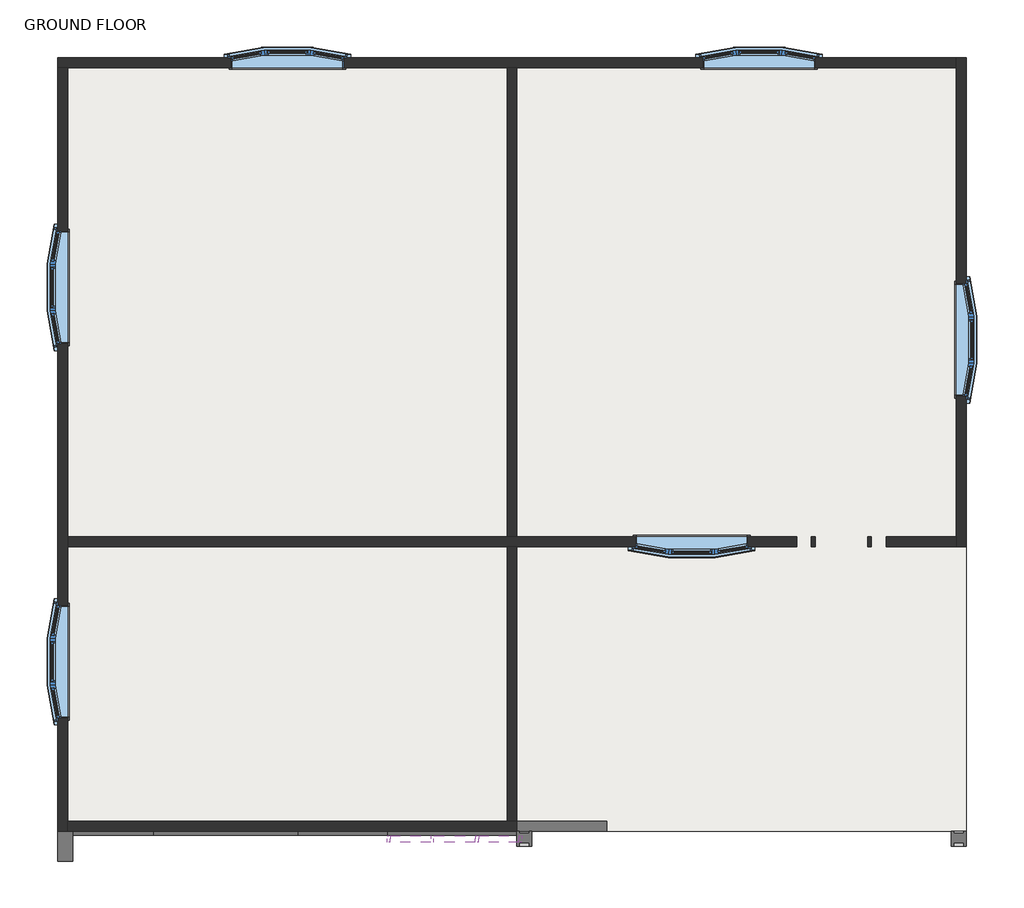
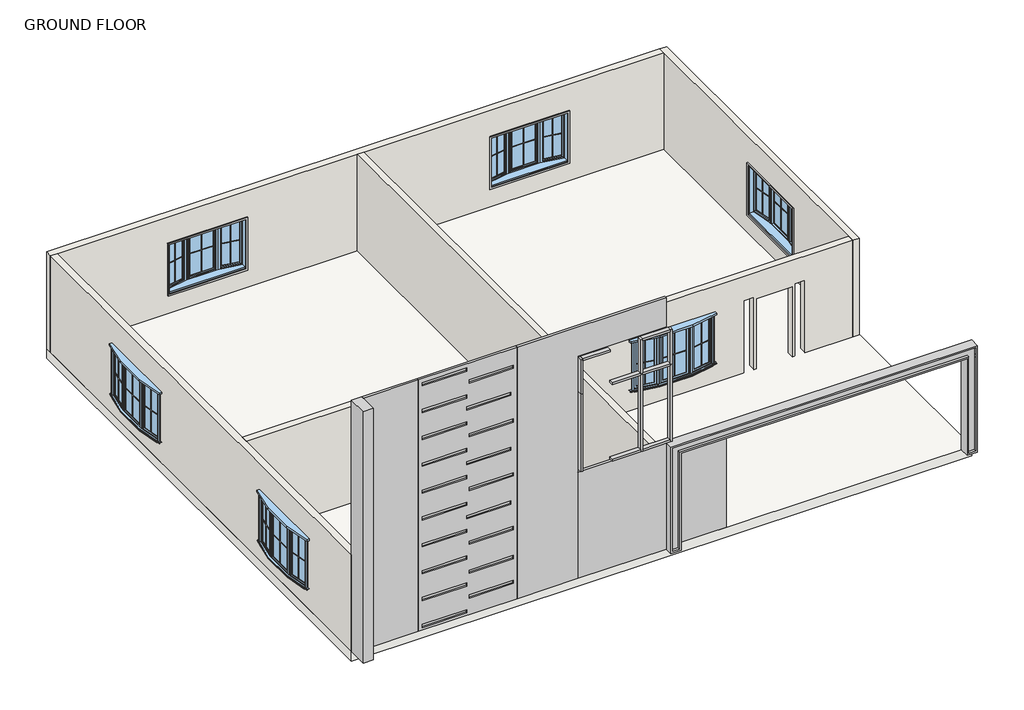
# One storey, incomplete: 31 proxies, 12 members, 7 walls, 6 windows, 1 slab.
"""IFC4 building model written with IfcOpenShell, lengths in millimetres."""

from ifc_helpers import new_model, si_unit, frame, origin, origin_with_axes, place, context, project, spatial, polyline, outline, extrude, faceted_brep, transform, mapped, element, save
from components import generic_models_1_generic_models_1_d450fbd8, generic_models_3_generic_models_3_9b1755e3, generic_models_4_generic_models_4_91b2e968, generic_models_5_generic_models_5_f46b040b, generic_models_6_generic_models_6_d33aa09a, generic_models_7_generic_models_7_539d4222, generic_models_8_generic_models_8_98324a9d, muntin_pattern_2x2_muntin_pattern_2x2_d8607f27, muntin_pattern_2x2_muntin_pattern_2x2_395d1e8c, trim_window_interior_flat_picture_frame_9ca7b173, member_f0fea5a5, member_ee409385, member_b90701c7, member_3972cc06, member_bef5179f, member_a085fe98, member_9b18e963, member_95153237, window_3790adff

model = new_model("IFC4")

# Units and contexts
model_context = context("Model", 3, world=origin())
ifc_project = project(units=[si_unit("LENGTHUNIT", "METRE", prefix="MILLI")], contexts=[model_context])

# Site, building, storey
site = spatial("IfcSite", under=ifc_project)
building = spatial("IfcBuilding", under=site)
storey = spatial("IfcBuildingStorey", under=building, Name="GROUND FLOOR", Elevation=0.0)

# Proxies
placement = place(None, origin())
generic_models_1_generic_models_1_shape = generic_models_1_generic_models_1_d450fbd8(model_context)
element("IfcBuildingElementProxy", 1, Name="Generic Models 1 : Generic Models 1", ObjectType="Generic Models 1 : Generic Models 1", at=placement, inside=storey, context=model_context, shape_type="MappedRepresentation", body=[
    mapped(generic_models_1_generic_models_1_shape, transform((0.0, 0.0, 0.0), x_axis=(1.0, 0.0, 0.0), y_axis=(0.0, 1.0, 0.0), z_axis=(0.0, 0.0, 1.0))),
])
generic_models_3_generic_models_3_shape = generic_models_3_generic_models_3_9b1755e3(model_context)
element("IfcBuildingElementProxy", 2, Name="Generic Models 3 : Generic Models 3", ObjectType="Generic Models 3 : Generic Models 3", at=placement, inside=storey, context=model_context, shape_type="MappedRepresentation", body=[
    mapped(generic_models_3_generic_models_3_shape, transform((0.0, 0.0, 0.0), x_axis=(1.0, 0.0, 0.0), y_axis=(0.0, 1.0, 0.0), z_axis=(0.0, 0.0, 1.0))),
])
generic_models_4_generic_models_4_shape = generic_models_4_generic_models_4_91b2e968(model_context)
element("IfcBuildingElementProxy", 3, Name="Generic Models 4 : Generic Models 4", ObjectType="Generic Models 4 : Generic Models 4", at=placement, inside=storey, context=model_context, shape_type="MappedRepresentation", body=[
    mapped(generic_models_4_generic_models_4_shape, transform((0.0, 0.0, 0.0), x_axis=(1.0, 0.0, 0.0), y_axis=(0.0, 1.0, 0.0), z_axis=(0.0, 0.0, 1.0))),
])
generic_models_5_generic_models_5_shape = generic_models_5_generic_models_5_f46b040b(model_context)
element("IfcBuildingElementProxy", 4, Name="Generic Models 5 : Generic Models 5", ObjectType="Generic Models 5 : Generic Models 5", at=placement, inside=storey, context=model_context, shape_type="MappedRepresentation", body=[
    mapped(generic_models_5_generic_models_5_shape, transform((0.0, 0.0, 0.0), x_axis=(1.0, 0.0, 0.0), y_axis=(0.0, 1.0, 0.0), z_axis=(0.0, 0.0, 1.0))),
])
generic_models_6_generic_models_6_shape = generic_models_6_generic_models_6_d33aa09a(model_context)
element("IfcBuildingElementProxy", 5, Name="Generic Models 6 : Generic Models 6", ObjectType="Generic Models 6 : Generic Models 6", at=placement, inside=storey, context=model_context, shape_type="MappedRepresentation", body=[
    mapped(generic_models_6_generic_models_6_shape, transform((0.0, 0.0, 0.0), x_axis=(1.0, 0.0, 0.0), y_axis=(0.0, 1.0, 0.0), z_axis=(0.0, 0.0, 1.0))),
])
generic_models_7_generic_models_7_shape = generic_models_7_generic_models_7_539d4222(model_context)
element("IfcBuildingElementProxy", 6, Name="Generic Models 7 : Generic Models 7", ObjectType="Generic Models 7 : Generic Models 7", at=placement, inside=storey, context=model_context, shape_type="MappedRepresentation", body=[
    mapped(generic_models_7_generic_models_7_shape, transform((0.0, 0.0, 0.0), x_axis=(1.0, 0.0, 0.0), y_axis=(0.0, 1.0, 0.0), z_axis=(0.0, 0.0, 1.0))),
])
generic_models_8_generic_models_8_shape = generic_models_8_generic_models_8_98324a9d(model_context)
element("IfcBuildingElementProxy", 7, Name="Generic Models 8 : Generic Models 8", ObjectType="Generic Models 8 : Generic Models 8", at=placement, inside=storey, context=model_context, shape_type="MappedRepresentation", body=[
    mapped(generic_models_8_generic_models_8_shape, transform((0.0, 0.0, 0.0), x_axis=(1.0, 0.0, 0.0), y_axis=(0.0, 1.0, 0.0), z_axis=(0.0, 0.0, 1.0))),
])
muntin_pattern_2x2_muntin_pattern_2x2_shape = muntin_pattern_2x2_muntin_pattern_2x2_d8607f27(model_context)
element("IfcBuildingElementProxy", 8, Name="Muntin Pattern_2x2 : Muntin Pattern_2x2", ObjectType="Muntin Pattern_2x2 : Muntin Pattern_2x2", at=placement, inside=storey, context=model_context, shape_type="MappedRepresentation", body=[
    mapped(muntin_pattern_2x2_muntin_pattern_2x2_shape, transform((4145.554407, 1568.600611, 730.25), x_axis=(-1.0, 0.0, 0.0), y_axis=(0.0, -1.0, 0.0), z_axis=(0.0, 0.0, 1.0))),
])
element("IfcBuildingElementProxy", 9, Name="Muntin Pattern_2x2 : Muntin Pattern_2x2", ObjectType="Muntin Pattern_2x2 : Muntin Pattern_2x2", at=placement, inside=storey, context=model_context, shape_type="MappedRepresentation", body=[
    mapped(muntin_pattern_2x2_muntin_pattern_2x2_shape, transform((9844.679407, 5896.125611, 730.25), x_axis=(0.0, -1.0, 0.0), y_axis=(1.0, 0.0, 0.0), z_axis=(0.0, 0.0, 1.0))),
])
element("IfcBuildingElementProxy", 10, Name="Muntin Pattern_2x2 : Muntin Pattern_2x2", ObjectType="Muntin Pattern_2x2 : Muntin Pattern_2x2", at=placement, inside=storey, context=model_context, shape_type="MappedRepresentation", body=[
    mapped(muntin_pattern_2x2_muntin_pattern_2x2_shape, transform((-4084.045593, 11747.650611, 730.25), x_axis=(1.0, 0.0, 0.0), y_axis=(0.0, 1.0, 0.0), z_axis=(0.0, 0.0, 1.0))),
])
element("IfcBuildingElementProxy", 11, Name="Muntin Pattern_2x2 : Muntin Pattern_2x2", ObjectType="Muntin Pattern_2x2 : Muntin Pattern_2x2", at=placement, inside=storey, context=model_context, shape_type="MappedRepresentation", body=[
    mapped(muntin_pattern_2x2_muntin_pattern_2x2_shape, transform((5517.154407, 11747.650611, 730.25), x_axis=(1.0, 0.0, 0.0), y_axis=(0.0, 1.0, 0.0), z_axis=(0.0, 0.0, 1.0))),
])
element("IfcBuildingElementProxy", 12, Name="Muntin Pattern_2x2 : Muntin Pattern_2x2", ObjectType="Muntin Pattern_2x2 : Muntin Pattern_2x2", at=placement, inside=storey, context=model_context, shape_type="MappedRepresentation", body=[
    mapped(muntin_pattern_2x2_muntin_pattern_2x2_shape, transform((-8868.770593, 6962.925611, 730.25), x_axis=(0.0, 1.0, 0.0), y_axis=(-1.0, 0.0, 0.0), z_axis=(0.0, 0.0, 1.0))),
])
element("IfcBuildingElementProxy", 13, Name="Muntin Pattern_2x2 : Muntin Pattern_2x2", ObjectType="Muntin Pattern_2x2 : Muntin Pattern_2x2", at=placement, inside=storey, context=model_context, shape_type="MappedRepresentation", body=[
    mapped(muntin_pattern_2x2_muntin_pattern_2x2_shape, transform((-8868.770593, -657.074389, 730.25), x_axis=(0.0, 1.0, 0.0), y_axis=(-1.0, 0.0, 0.0), z_axis=(0.0, 0.0, 1.0))),
])
muntin_pattern_2x2_muntin_pattern_2x2_2_shape = muntin_pattern_2x2_muntin_pattern_2x2_395d1e8c(model_context)
element("IfcBuildingElementProxy", 14, Name="Muntin Pattern_2x2 : Muntin Pattern_2x2", ObjectType="Muntin Pattern_2x2 : Muntin Pattern_2x2", at=placement, inside=storey, context=model_context, shape_type="MappedRepresentation", body=[
    mapped(muntin_pattern_2x2_muntin_pattern_2x2_2_shape, transform((4981.9237745, 1633.1915685, 730.25), x_axis=(-0.9848077530122097, -0.1736481776669209, 0.0), y_axis=(0.1736481776669209, -0.9848077530122097, 0.0), z_axis=(0.0, 0.0, 1.0))),
])
element("IfcBuildingElementProxy", 15, Name="Muntin Pattern_2x2 : Muntin Pattern_2x2", ObjectType="Muntin Pattern_2x2 : Muntin Pattern_2x2", at=placement, inside=storey, context=model_context, shape_type="MappedRepresentation", body=[
    mapped(muntin_pattern_2x2_muntin_pattern_2x2_2_shape, transform((3309.1850396, 1633.1915685, 730.25), x_axis=(-0.9848077530122065, 0.17364817766693977, 0.0), y_axis=(-0.17364817766693977, -0.9848077530122065, 0.0), z_axis=(0.0, 0.0, 1.0))),
])
element("IfcBuildingElementProxy", 16, Name="Muntin Pattern_2x2 : Muntin Pattern_2x2", ObjectType="Muntin Pattern_2x2 : Muntin Pattern_2x2", at=placement, inside=storey, context=model_context, shape_type="MappedRepresentation", body=[
    mapped(muntin_pattern_2x2_muntin_pattern_2x2_2_shape, transform((9780.0884495, 6732.4949785, 730.25), x_axis=(0.1736481776669241, -0.9848077530122091, 0.0), y_axis=(0.9848077530122091, 0.1736481776669241, 0.0), z_axis=(0.0, 0.0, 1.0))),
])
element("IfcBuildingElementProxy", 17, Name="Muntin Pattern_2x2 : Muntin Pattern_2x2", ObjectType="Muntin Pattern_2x2 : Muntin Pattern_2x2", at=placement, inside=storey, context=model_context, shape_type="MappedRepresentation", body=[
    mapped(muntin_pattern_2x2_muntin_pattern_2x2_2_shape, transform((9780.0884495, 5059.7562435, 730.25), x_axis=(-0.17364817766693658, -0.984807753012207, 0.0), y_axis=(0.984807753012207, -0.17364817766693658, 0.0), z_axis=(0.0, 0.0, 1.0))),
])
element("IfcBuildingElementProxy", 18, Name="Muntin Pattern_2x2 : Muntin Pattern_2x2", ObjectType="Muntin Pattern_2x2 : Muntin Pattern_2x2", at=placement, inside=storey, context=model_context, shape_type="MappedRepresentation", body=[
    mapped(muntin_pattern_2x2_muntin_pattern_2x2_2_shape, transform((-4920.4149604, 11683.0596534, 730.25), x_axis=(0.9848077530122091, 0.1736481776669241, 0.0), y_axis=(-0.1736481776669241, 0.9848077530122091, 0.0), z_axis=(0.0, 0.0, 1.0))),
])
element("IfcBuildingElementProxy", 19, Name="Muntin Pattern_2x2 : Muntin Pattern_2x2", ObjectType="Muntin Pattern_2x2 : Muntin Pattern_2x2", at=placement, inside=storey, context=model_context, shape_type="MappedRepresentation", body=[
    mapped(muntin_pattern_2x2_muntin_pattern_2x2_2_shape, transform((-3247.6762255, 11683.0596534, 730.25), x_axis=(0.984807753012207, -0.17364817766693658, 0.0), y_axis=(0.17364817766693658, 0.984807753012207, 0.0), z_axis=(0.0, 0.0, 1.0))),
])
element("IfcBuildingElementProxy", 20, Name="Muntin Pattern_2x2 : Muntin Pattern_2x2", ObjectType="Muntin Pattern_2x2 : Muntin Pattern_2x2", at=placement, inside=storey, context=model_context, shape_type="MappedRepresentation", body=[
    mapped(muntin_pattern_2x2_muntin_pattern_2x2_2_shape, transform((4680.7850396, 11683.0596534, 730.25), x_axis=(0.9848077530122091, 0.1736481776669241, 0.0), y_axis=(-0.1736481776669241, 0.9848077530122091, 0.0), z_axis=(0.0, 0.0, 1.0))),
])
element("IfcBuildingElementProxy", 21, Name="Muntin Pattern_2x2 : Muntin Pattern_2x2", ObjectType="Muntin Pattern_2x2 : Muntin Pattern_2x2", at=placement, inside=storey, context=model_context, shape_type="MappedRepresentation", body=[
    mapped(muntin_pattern_2x2_muntin_pattern_2x2_2_shape, transform((6353.5237745, 11683.0596534, 730.25), x_axis=(0.984807753012207, -0.17364817766693658, 0.0), y_axis=(0.17364817766693658, 0.984807753012207, 0.0), z_axis=(0.0, 0.0, 1.0))),
])
element("IfcBuildingElementProxy", 22, Name="Muntin Pattern_2x2 : Muntin Pattern_2x2", ObjectType="Muntin Pattern_2x2 : Muntin Pattern_2x2", at=placement, inside=storey, context=model_context, shape_type="MappedRepresentation", body=[
    mapped(muntin_pattern_2x2_muntin_pattern_2x2_2_shape, transform((-8804.1796354, 6126.5562435, 730.25), x_axis=(-0.1736481776669241, 0.9848077530122091, 0.0), y_axis=(-0.9848077530122091, -0.1736481776669241, 0.0), z_axis=(0.0, 0.0, 1.0))),
])
element("IfcBuildingElementProxy", 23, Name="Muntin Pattern_2x2 : Muntin Pattern_2x2", ObjectType="Muntin Pattern_2x2 : Muntin Pattern_2x2", at=placement, inside=storey, context=model_context, shape_type="MappedRepresentation", body=[
    mapped(muntin_pattern_2x2_muntin_pattern_2x2_2_shape, transform((-8804.1796354, 7799.2949785, 730.25), x_axis=(0.17364817766693658, 0.984807753012207, 0.0), y_axis=(-0.984807753012207, 0.17364817766693658, 0.0), z_axis=(0.0, 0.0, 1.0))),
])
element("IfcBuildingElementProxy", 24, Name="Muntin Pattern_2x2 : Muntin Pattern_2x2", ObjectType="Muntin Pattern_2x2 : Muntin Pattern_2x2", at=placement, inside=storey, context=model_context, shape_type="MappedRepresentation", body=[
    mapped(muntin_pattern_2x2_muntin_pattern_2x2_2_shape, transform((-8804.1796354, -1493.4437565, 730.25), x_axis=(-0.1736481776669241, 0.9848077530122091, 0.0), y_axis=(-0.9848077530122091, -0.1736481776669241, 0.0), z_axis=(0.0, 0.0, 1.0))),
])
element("IfcBuildingElementProxy", 25, Name="Muntin Pattern_2x2 : Muntin Pattern_2x2", ObjectType="Muntin Pattern_2x2 : Muntin Pattern_2x2", at=placement, inside=storey, context=model_context, shape_type="MappedRepresentation", body=[
    mapped(muntin_pattern_2x2_muntin_pattern_2x2_2_shape, transform((-8804.1796354, 179.2949785, 730.25), x_axis=(0.17364817766693658, 0.984807753012207, 0.0), y_axis=(-0.984807753012207, 0.17364817766693658, 0.0), z_axis=(0.0, 0.0, 1.0))),
])
trim_window_interior_flat_picture_frame_shape = trim_window_interior_flat_picture_frame_9ca7b173(model_context)
element("IfcBuildingElementProxy", 26, Name="Trim-Window-Interior-Flat : Picture Frame", ObjectType="Trim-Window-Interior-Flat : Picture Frame", at=placement, inside=storey, context=model_context, shape_type="MappedRepresentation", body=[
    mapped(trim_window_interior_flat_picture_frame_shape, transform((4145.554407, 1882.925611, 2184.4), x_axis=(-1.0, 0.0, 0.0), y_axis=(0.0, 0.0, 1.0), z_axis=(0.0, 1.0, 0.0))),
])
element("IfcBuildingElementProxy", 27, Name="Trim-Window-Interior-Flat : Picture Frame", ObjectType="Trim-Window-Interior-Flat : Picture Frame", at=placement, inside=storey, context=model_context, shape_type="MappedRepresentation", body=[
    mapped(trim_window_interior_flat_picture_frame_shape, transform((9530.354407, 5896.125611, 2184.4), x_axis=(0.0, -1.0, 0.0), y_axis=(0.0, 0.0, 1.0), z_axis=(-1.0, 0.0, 0.0))),
])
element("IfcBuildingElementProxy", 28, Name="Trim-Window-Interior-Flat : Picture Frame", ObjectType="Trim-Window-Interior-Flat : Picture Frame", at=placement, inside=storey, context=model_context, shape_type="MappedRepresentation", body=[
    mapped(trim_window_interior_flat_picture_frame_shape, transform((-4084.045593, 11433.325611, 2184.4), x_axis=(1.0, 0.0, 0.0), y_axis=(0.0, 0.0, 1.0), z_axis=(0.0, -1.0, 0.0))),
])
element("IfcBuildingElementProxy", 29, Name="Trim-Window-Interior-Flat : Picture Frame", ObjectType="Trim-Window-Interior-Flat : Picture Frame", at=placement, inside=storey, context=model_context, shape_type="MappedRepresentation", body=[
    mapped(trim_window_interior_flat_picture_frame_shape, transform((5517.154407, 11433.325611, 2184.4), x_axis=(1.0, 0.0, 0.0), y_axis=(0.0, 0.0, 1.0), z_axis=(0.0, -1.0, 0.0))),
])
element("IfcBuildingElementProxy", 30, Name="Trim-Window-Interior-Flat : Picture Frame", ObjectType="Trim-Window-Interior-Flat : Picture Frame", at=placement, inside=storey, context=model_context, shape_type="MappedRepresentation", body=[
    mapped(trim_window_interior_flat_picture_frame_shape, transform((-8554.445593, 6962.925611, 2184.4), x_axis=(0.0, 1.0, 0.0), y_axis=(0.0, 0.0, 1.0), z_axis=(1.0, 0.0, 0.0))),
])
element("IfcBuildingElementProxy", 31, Name="Trim-Window-Interior-Flat : Picture Frame", ObjectType="Trim-Window-Interior-Flat : Picture Frame", at=placement, inside=storey, context=model_context, shape_type="MappedRepresentation", body=[
    mapped(trim_window_interior_flat_picture_frame_shape, transform((-8554.445593, -657.074389, 2184.4), x_axis=(0.0, 1.0, 0.0), y_axis=(0.0, 0.0, 1.0), z_axis=(1.0, 0.0, 0.0))),
])

# Members
member_shape = member_f0fea5a5(model_context)
element("IfcMember", 32, ObjectType="Rectangular Mullion : 2.5\" x 5\" rectangular", at=placement, inside=storey, context=model_context, shape_type="MappedRepresentation", body=[
    mapped(member_shape, transform((-223.2455734, -4263.874389, 3450.2081328), x_axis=(-1.0, 0.0, 0.0), y_axis=(0.0, 1.0, 0.0), z_axis=(0.0, 0.0, -1.0))),
])
member_2_shape = member_ee409385(model_context)
element("IfcMember", 33, ObjectType="Rectangular Mullion : 2.5\" x 5\" rectangular", at=placement, inside=storey, context=model_context, shape_type="MappedRepresentation", body=[
    mapped(member_2_shape, transform((-2052.0455733, -4263.874389, 3450.2081328), x_axis=(-1.0, 0.0, 0.0), y_axis=(0.0, 1.0, 0.0), z_axis=(0.0, 0.0, -1.0))),
])
element("IfcMember", 34, ObjectType="Rectangular Mullion : 2.5\" x 5\" rectangular", at=placement, inside=storey, context=model_context, shape_type="MappedRepresentation", body=[
    mapped(member_2_shape, transform((691.1544267, -4263.874389, 5888.6081328), x_axis=(1.0, 0.0, 0.0), y_axis=(0.0, 1.0, 0.0), z_axis=(0.0, 0.0, 1.0))),
])
member_3_shape = member_b90701c7(model_context)
element("IfcMember", 35, ObjectType="Rectangular Mullion : 2.5\" x 5\" rectangular", at=placement, inside=storey, context=model_context, shape_type="MappedRepresentation", body=[
    mapped(member_3_shape, transform((-223.2455734, -4263.874389, 5888.6081328), x_axis=(-1.0, 0.0, 0.0), y_axis=(0.0, 1.0, 0.0), z_axis=(0.0, 0.0, -1.0))),
])
member_4_shape = member_3972cc06(model_context)
element("IfcMember", 36, ObjectType="Rectangular Mullion : 2.5\" x 5\" rectangular", at=placement, inside=storey, context=model_context, shape_type="MappedRepresentation", body=[
    mapped(member_4_shape, transform((-2052.0455733, -4263.874389, 5888.6081328), x_axis=(-1.0, 0.0, 0.0), y_axis=(0.0, 1.0, 0.0), z_axis=(0.0, 0.0, -1.0))),
])
element("IfcMember", 37, ObjectType="Rectangular Mullion : 2.5\" x 5\" rectangular", at=placement, inside=storey, context=model_context, shape_type="MappedRepresentation", body=[
    mapped(member_4_shape, transform((691.1544267, -4263.874389, 6988.1851727), x_axis=(1.0, 0.0, 0.0), y_axis=(0.0, 1.0, 0.0), z_axis=(0.0, 0.0, 1.0))),
])
member_5_shape = member_bef5179f(model_context)
element("IfcMember", 38, ObjectType="Rectangular Mullion : 2.5\" x 5\" rectangular", at=placement, inside=storey, context=model_context, shape_type="MappedRepresentation", body=[
    mapped(member_5_shape, transform((-1988.5455733, -4263.874389, 6988.1851727), x_axis=(0.0, 0.0, 1.0), y_axis=(0.0, 1.0, 0.0), z_axis=(-1.0, 0.0, 0.0))),
])
element("IfcMember", 39, ObjectType="Rectangular Mullion : 2.5\" x 5\" rectangular", at=placement, inside=storey, context=model_context, shape_type="MappedRepresentation", body=[
    mapped(member_5_shape, transform((-191.4955734, -4263.874389, 6988.1851727), x_axis=(0.0, 0.0, 1.0), y_axis=(0.0, 1.0, 0.0), z_axis=(-1.0, 0.0, 0.0))),
])
element("IfcMember", 40, ObjectType="Rectangular Mullion : 2.5\" x 5\" rectangular", at=placement, inside=storey, context=model_context, shape_type="MappedRepresentation", body=[
    mapped(member_5_shape, transform((627.6544267, -4263.874389, 3450.2081328), x_axis=(0.0, 0.0, -1.0), y_axis=(0.0, 1.0, 0.0), z_axis=(1.0, 0.0, 0.0))),
])
member_6_shape = member_a085fe98(model_context)
element("IfcMember", 41, ObjectType="Rectangular Mullion : 2.5\" x 5\" rectangular", at=placement, inside=storey, context=model_context, shape_type="MappedRepresentation", body=[
    mapped(member_6_shape, transform((-191.4955734, -4263.874389, 5888.6081328), x_axis=(0.0, 0.0, 1.0), y_axis=(0.0, 1.0, 0.0), z_axis=(-1.0, 0.0, 0.0))),
])
member_7_shape = member_9b18e963(model_context)
element("IfcMember", 42, ObjectType="Rectangular Mullion : 2.5\" x 5\" rectangular", at=placement, inside=storey, context=model_context, shape_type="MappedRepresentation", body=[
    mapped(member_7_shape, transform((-254.9955734, -4263.874389, 3450.2081328), x_axis=(0.0, 0.0, -1.0), y_axis=(0.0, 1.0, 0.0), z_axis=(1.0, 0.0, 0.0))),
])
member_8_shape = member_95153237(model_context)
element("IfcMember", 43, ObjectType="Rectangular Mullion : 2.5\" x 5\" rectangular", at=placement, inside=storey, context=model_context, shape_type="MappedRepresentation", body=[
    mapped(member_8_shape, transform((-1105.8955732, -4263.874389, 5888.6081328), x_axis=(0.0, 0.0, 1.0), y_axis=(0.0, 1.0, 0.0), z_axis=(-1.0, 0.0, 0.0))),
])

# Slab
element("IfcSlab", 44, ObjectType="Generic - 12\"", at=placement, inside=storey, context=model_context, shape_type="SweptSolid", body=[
    extrude(outline(polyline([(9733.554407, 11636.525611), (9733.554407, -4111.474389), (-8757.645593, -4111.474389), (-8757.645593, 11636.525611), (9733.554407, 11636.525611)])), frame((0.0, 0.0, -304.8), z_axis=(0.0, 0.0, 1.0), x_axis=(1.0, 0.0, 0.0)), (0.0, 0.0, 1.0), 304.8),
])

# Walls
element("IfcWall", 45, ObjectType="Generic - 8\"", at=placement, inside=storey, context=model_context, shape_type="Brep", body=[
    faceted_brep([(-8757.645593, 11433.325611, 0.0), (-8554.445593, 11433.325611, 0.0), (386.354407, 11433.325611, 0.0), (589.554407, 11433.325611, 0.0), (9530.354407, 11433.325611, 0.0), (9530.354407, 11433.325611, 3048.0), (589.554407, 11433.325611, 3048.0), (386.354407, 11433.325611, 3048.0), (-8554.445593, 11433.325611, 3048.0), (-8757.645593, 11433.325611, 3048.0), (-5227.045593, 11433.325611, 2184.4), (-2941.045593, 11433.325611, 2184.4), (-2941.045593, 11433.325611, 609.6), (-5227.045593, 11433.325611, 609.6), (4374.154407, 11433.325611, 2184.4), (6660.154407, 11433.325611, 2184.4), (6660.154407, 11433.325611, 609.6), (4374.154407, 11433.325611, 609.6), (-8757.645593, 11636.525611, 0.0), (-8757.645593, 11636.525611, 3048.0), (9530.354407, 11636.525611, 3048.0), (9530.354407, 11636.525611, 0.0), (-2928.9162677, 11636.525611, 2184.4), (-5239.1749182, 11636.525611, 2184.4), (-5239.1749182, 11636.525611, 609.6), (-2928.9162677, 11636.525611, 609.6), (6672.2837323, 11636.525611, 2184.4), (4362.0250818, 11636.525611, 2184.4), (4362.0250818, 11636.525611, 609.6), (6672.2837323, 11636.525611, 609.6), (-5227.045593, 11567.7367894, 2184.4), (-2941.045593, 11567.7367894, 2184.4), (-5227.045593, 11567.7367894, 609.6), (-2941.045593, 11567.7367894, 609.6), (4374.154407, 11567.7367894, 2184.4), (6660.154407, 11567.7367894, 2184.4), (4374.154407, 11567.7367894, 609.6), (6660.154407, 11567.7367894, 609.6)], [[[0, 1, 2, 3, 4, 5, 6, 7, 8, 9], [10, 11, 12, 13], [14, 15, 16, 17]], [[18, 19, 20, 21], [22, 23, 24, 25], [26, 27, 28, 29]], [[4, 3, 2, 1, 0, 18, 21]], [[0, 9, 19, 18]], [[5, 4, 21, 20]], [[9, 8, 7, 6, 5, 20, 19]], [[30, 23, 22, 31, 11, 10]], [[32, 13, 12, 33, 25, 24]], [[30, 10, 13, 32]], [[11, 31, 33, 12]], [[31, 22, 25, 33]], [[23, 30, 32, 24]], [[34, 27, 26, 35, 15, 14]], [[36, 17, 16, 37, 29, 28]], [[34, 14, 17, 36]], [[15, 35, 37, 16]], [[35, 26, 29, 37]], [[27, 34, 36, 28]]]),
])
element("IfcWall", 46, ObjectType="Generic - 8\"", at=placement, inside=storey, context=model_context, shape_type="Brep", body=[
    faceted_brep([(-8554.445593, -4111.474389, 0.0), (-8554.445593, -3908.274389, 0.0), (-8554.445593, 1679.725611, 0.0), (-8554.445593, 1882.925611, 0.0), (-8554.445593, 11433.325611, 0.0), (-8554.445593, 11433.325611, 3048.0), (-8554.445593, 1882.925611, 3048.0), (-8554.445593, 1679.725611, 3048.0), (-8554.445593, -3908.274389, 3048.0), (-8554.445593, -4111.474389, 3048.0), (-8554.445593, 5819.925611, 2184.4), (-8554.445593, 8105.925611, 2184.4), (-8554.445593, 8105.925611, 609.6), (-8554.445593, 5819.925611, 609.6), (-8554.445593, -1800.074389, 2184.4), (-8554.445593, 485.925611, 2184.4), (-8554.445593, 485.925611, 609.6), (-8554.445593, -1800.074389, 609.6), (-8757.645593, -4111.474389, 0.0), (-8757.645593, -4111.474389, 3048.0), (-8757.645593, 11433.325611, 3048.0), (-8757.645593, 11433.325611, 0.0), (-8757.645593, 8118.0549362, 2184.4), (-8757.645593, 5807.7962858, 2184.4), (-8757.645593, 5807.7962858, 609.6), (-8757.645593, 8118.0549362, 609.6), (-8757.645593, 498.0549362, 2184.4), (-8757.645593, -1812.2037142, 2184.4), (-8757.645593, -1812.2037142, 609.6), (-8757.645593, 498.0549362, 609.6), (-8688.8567714, 5819.925611, 2184.4), (-8688.8567714, 8105.925611, 2184.4), (-8688.8567714, 5819.925611, 609.6), (-8688.8567714, 8105.925611, 609.6), (-8688.8567714, -1800.074389, 2184.4), (-8688.8567714, 485.925611, 2184.4), (-8688.8567714, -1800.074389, 609.6), (-8688.8567714, 485.925611, 609.6)], [[[0, 1, 2, 3, 4, 5, 6, 7, 8, 9], [10, 11, 12, 13], [14, 15, 16, 17]], [[18, 19, 20, 21], [22, 23, 24, 25], [26, 27, 28, 29]], [[4, 3, 2, 1, 0, 18, 21]], [[0, 9, 19, 18]], [[5, 4, 21, 20]], [[9, 8, 7, 6, 5, 20, 19]], [[30, 23, 22, 31, 11, 10]], [[32, 13, 12, 33, 25, 24]], [[30, 10, 13, 32]], [[11, 31, 33, 12]], [[31, 22, 25, 33]], [[23, 30, 32, 24]], [[34, 27, 26, 35, 15, 14]], [[36, 17, 16, 37, 29, 28]], [[34, 14, 17, 36]], [[15, 35, 37, 16]], [[35, 26, 29, 37]], [[27, 34, 36, 28]]]),
])
element("IfcWall", 47, ObjectType="Generic - 8\"", at=placement, inside=storey, context=model_context, shape_type="Brep", body=[
    faceted_brep([(589.554407, -3908.274389, 0.0), (386.354407, -3908.274389, 0.0), (-8554.445593, -3908.274389, 0.0), (-8554.445593, -3908.274389, 3048.0), (386.354407, -3908.274389, 3048.0), (589.554407, -3908.274389, 3048.0), (589.554407, -4111.474389, 0.0), (589.554407, -4111.474389, 3048.0), (-8554.445593, -4111.474389, 3048.0), (-8554.445593, -4111.474389, 0.0)], [[[0, 1, 2, 3, 4, 5]], [[6, 7, 8, 9]], [[2, 1, 0, 6, 9]], [[3, 2, 9, 8]], [[0, 5, 7, 6]], [[5, 4, 3, 8, 7]]]),
])
element("IfcWall", 48, ObjectType="Generic - 8\"", at=placement, inside=storey, context=model_context, shape_type="Brep", body=[
    faceted_brep([(9530.354407, 11636.525611, 0.0), (9530.354407, 11433.325611, 0.0), (9530.354407, 1882.925611, 0.0), (9530.354407, 1679.725611, 0.0), (9530.354407, 1679.725611, 3048.0), (9530.354407, 1882.925611, 3048.0), (9530.354407, 11433.325611, 3048.0), (9530.354407, 11636.525611, 3048.0), (9530.354407, 7039.125611, 2184.4), (9530.354407, 4753.125611, 2184.4), (9530.354407, 4753.125611, 609.6), (9530.354407, 7039.125611, 609.6), (9733.554407, 11636.525611, 0.0), (9733.554407, 11636.525611, 3048.0), (9733.554407, 1679.725611, 3048.0), (9733.554407, 1679.725611, 0.0), (9733.554407, 4740.9962858, 2184.4), (9733.554407, 7051.2549362, 2184.4), (9733.554407, 7051.2549362, 609.6), (9733.554407, 4740.9962858, 609.6), (9664.7655855, 7039.125611, 2184.4), (9664.7655855, 4753.125611, 2184.4), (9664.7655855, 7039.125611, 609.6), (9664.7655855, 4753.125611, 609.6)], [[[0, 1, 2, 3, 4, 5, 6, 7], [8, 9, 10, 11]], [[12, 13, 14, 15], [16, 17, 18, 19]], [[3, 2, 1, 0, 12, 15]], [[0, 7, 13, 12]], [[4, 3, 15, 14]], [[7, 6, 5, 4, 14, 13]], [[20, 17, 16, 21, 9, 8]], [[22, 11, 10, 23, 19, 18]], [[20, 8, 11, 22]], [[9, 21, 23, 10]], [[21, 16, 19, 23]], [[17, 20, 22, 18]]]),
])
element("IfcWall", 49, ObjectType="Generic - 8\"", at=placement, inside=storey, context=model_context, shape_type="Brep", body=[
    faceted_brep([(-8554.445593, 1679.725611, 3048.0), (-8554.445593, 1679.725611, 0.0), (386.354407, 1679.725611, 0.0), (589.554407, 1679.725611, 0.0), (6279.154407, 1679.725611, 0.0), (6279.154407, 1679.725611, 2286.0), (6583.954407, 1679.725611, 2286.0), (6583.954407, 1679.725611, 0.0), (6660.154407, 1679.725611, 0.0), (6660.154407, 1679.725611, 2209.8), (7726.954407, 1679.725611, 2209.8), (7726.954407, 1679.725611, 0.0), (7803.154407, 1679.725611, 0.0), (7803.154407, 1679.725611, 2286.0), (8107.954407, 1679.725611, 2286.0), (8107.954407, 1679.725611, 0.0), (9530.354407, 1679.725611, 0.0), (9530.354407, 1679.725611, 3048.0), (589.554407, 1679.725611, 3048.0), (386.354407, 1679.725611, 3048.0), (2990.4250818, 1679.725611, 2184.4), (5300.6837323, 1679.725611, 2184.4), (5300.6837323, 1679.725611, 609.6), (2990.4250818, 1679.725611, 609.6), (-8554.445593, 1882.925611, 0.0), (-8554.445593, 1882.925611, 3048.0), (386.354407, 1882.925611, 3048.0), (589.554407, 1882.925611, 3048.0), (9530.354407, 1882.925611, 3048.0), (9530.354407, 1882.925611, 0.0), (8107.954407, 1882.925611, 0.0), (8107.954407, 1882.925611, 2286.0), (7803.154407, 1882.925611, 2286.0), (7803.154407, 1882.925611, 0.0), (7726.954407, 1882.925611, 0.0), (7726.954407, 1882.925611, 2209.8), (6660.154407, 1882.925611, 2209.8), (6660.154407, 1882.925611, 0.0), (6583.954407, 1882.925611, 0.0), (6583.954407, 1882.925611, 2286.0), (6279.154407, 1882.925611, 2286.0), (6279.154407, 1882.925611, 0.0), (589.554407, 1882.925611, 0.0), (386.354407, 1882.925611, 0.0), (5288.554407, 1882.925611, 2184.4), (3002.554407, 1882.925611, 2184.4), (3002.554407, 1882.925611, 609.6), (5288.554407, 1882.925611, 609.6), (5288.554407, 1748.5144325, 2184.4), (3002.554407, 1748.5144325, 2184.4), (5288.554407, 1748.5144325, 609.6), (3002.554407, 1748.5144325, 609.6)], [[[0, 1, 2, 3, 4, 5, 6, 7, 8, 9, 10, 11, 12, 13, 14, 15, 16, 17, 18, 19], [20, 21, 22, 23]], [[24, 25, 26, 27, 28, 29, 30, 31, 32, 33, 34, 35, 36, 37, 38, 39, 40, 41, 42, 43], [44, 45, 46, 47]], [[1, 24, 43, 42, 41, 4, 3, 2]], [[29, 16, 15, 30]], [[37, 8, 7, 38]], [[11, 34, 33, 12]], [[1, 0, 25, 24]], [[17, 16, 29, 28]], [[0, 19, 18, 17, 28, 27, 26, 25]], [[36, 9, 8, 37]], [[9, 36, 35, 10]], [[10, 35, 34, 11]], [[33, 32, 13, 12]], [[31, 30, 15, 14]], [[32, 31, 14, 13]], [[41, 40, 5, 4]], [[39, 38, 7, 6]], [[40, 39, 6, 5]], [[48, 21, 20, 49, 45, 44]], [[50, 47, 46, 51, 23, 22]], [[48, 44, 47, 50]], [[45, 49, 51, 46]], [[49, 20, 23, 51]], [[21, 48, 50, 22]]]),
])
element("IfcWall", 50, ObjectType="Generic - 8\"", at=placement, inside=storey, context=model_context, shape_type="SweptSolid", body=[
    extrude(outline(polyline([(386.354407, 1882.925611), (386.354407, 11433.325611), (589.554407, 11433.325611), (589.554407, 1882.925611), (386.354407, 1882.925611)])), origin_with_axes(), (0.0, 0.0, 1.0), 3048.0),
])
element("IfcWall", 51, ObjectType="Generic - 8\"", at=placement, inside=storey, context=model_context, shape_type="SweptSolid", body=[
    extrude(outline(polyline([(589.554407, 1679.725611), (589.554407, -3908.274389), (386.354407, -3908.274389), (386.354407, 1679.725611), (589.554407, 1679.725611)])), origin_with_axes(), (0.0, 0.0, 1.0), 3048.0),
])

# Windows
window_shape = window_3790adff(model_context)
element("IfcWindow", 52, ObjectType="Window-Bay-Casement-10_Degree_Angle : 90\" x 60\" x 6\"", at=placement, inside=storey, context=model_context, shape_type="MappedRepresentation", body=[
    mapped(window_shape, transform((4145.554407, 1781.325611, 0.0), x_axis=(-1.0, 0.0, 0.0), y_axis=(0.0, -1.0, 0.0), z_axis=(0.0, 0.0, 1.0))),
])
element("IfcWindow", 53, ObjectType="Window-Bay-Casement-10_Degree_Angle : 90\" x 60\" x 6\"", at=placement, inside=storey, context=model_context, shape_type="MappedRepresentation", body=[
    mapped(window_shape, transform((9631.954407, 5896.125611, 0.0), x_axis=(0.0, -1.0, 0.0), y_axis=(1.0, 0.0, 0.0), z_axis=(0.0, 0.0, 1.0))),
])
element("IfcWindow", 54, ObjectType="Window-Bay-Casement-10_Degree_Angle : 90\" x 60\" x 6\"", at=placement, inside=storey, context=model_context, shape_type="MappedRepresentation", body=[
    mapped(window_shape, transform((-4084.045593, 11534.925611, 0.0), x_axis=(1.0, 0.0, 0.0), y_axis=(0.0, 1.0, 0.0), z_axis=(0.0, 0.0, 1.0))),
])
element("IfcWindow", 55, ObjectType="Window-Bay-Casement-10_Degree_Angle : 90\" x 60\" x 6\"", at=placement, inside=storey, context=model_context, shape_type="MappedRepresentation", body=[
    mapped(window_shape, transform((5517.154407, 11534.925611, 0.0), x_axis=(1.0, 0.0, 0.0), y_axis=(0.0, 1.0, 0.0), z_axis=(0.0, 0.0, 1.0))),
])
element("IfcWindow", 56, ObjectType="Window-Bay-Casement-10_Degree_Angle : 90\" x 60\" x 6\"", at=placement, inside=storey, context=model_context, shape_type="MappedRepresentation", body=[
    mapped(window_shape, transform((-8656.045593, 6962.925611, 0.0), x_axis=(0.0, 1.0, 0.0), y_axis=(-1.0, 0.0, 0.0), z_axis=(0.0, 0.0, 1.0))),
])
element("IfcWindow", 57, ObjectType="Window-Bay-Casement-10_Degree_Angle : 90\" x 60\" x 6\"", at=placement, inside=storey, context=model_context, shape_type="MappedRepresentation", body=[
    mapped(window_shape, transform((-8656.045593, -657.074389, 0.0), x_axis=(0.0, 1.0, 0.0), y_axis=(-1.0, 0.0, 0.0), z_axis=(0.0, 0.0, 1.0))),
])

save(model, "model.ifc")

# Revit data of these elements
# Type "Muntin Pattern_2x2 : Muntin Pattern_2x2"
#   Width [instance default] = 4' - 0"
#   Thickness = 0' - 0 1/2"
#   Height [instance default] = 4' - 0"
#   Distance = 0' - 0 3/4"
#   Interior Material [instance default] = none
#   Exterior Material [instance default] = none
#   Default Elevation = 0
# Type "Trim-Window-Interior-Flat : Picture Frame"
#   Trim Thickness_Picture Frame = 0' - 1 1/4"
#   Trim Width = 0' - 2 1/4"
#   Trim Thickness_with Sill = 0' - 0 3/4"
#   Sill Thickness = 0' - 1 1/4"
#   Opening Width [instance default] = 2' - 0"
#   Opening Height [instance default] = 3' - 0"
#   Default Elevation = 4' - 0"
#   Sill = no
#   Picture Frame = yes
#   Trim Material [instance default] = none
# Type "Rectangular Mullion : 2.5\" x 5\" rectangular"
#   built-in parameter 1007304 = 0.416667 (stored number, unit not read)
#   built-in parameter 1007301 = 0.104167 (stored number, unit not read)
#   built-in parameter 1007300 = 0.104167 (stored number, unit not read)
# Type "Generic - 12\""
#   Assembly Code = "B1010"
#   Function = 0
#   Layers, outside or top first: 1' - 0" no material (function 1)
# Type "Generic - 8\""
#   Assembly Code = "B2010"
#   Layers, outside or top first: 0' - 8" no material (function 1)
# Type "Window-Bay-Casement-10_Degree_Angle : 90\" x 60\" x 6\""
#   Type Mark = "18"
#   Fire Rating = "0.5h"
#   Assembly Code = "B2020100"
#   Analytic Construction = "Double glazing - domestic"
#   Width of Middle Sash = 2' - 9.07789"
#   Width = 7' - 6"
#   Visual Light Transmittance = 0.81
#   Thermal Resistance (R) = 1.8146 (h·ft²·°F)/BTU
#   Solar Heat Gain Coefficient = 0.76
#   Rough Width = 7' - 6 1/2"
#   Rough Height = 5' - 0 1/2"
#   Length 4 = 0' - 0.24059"
#   Length 3 = 0' - 0 7/64"
#   Length 2 = 3' - 1.29661"
#   Length 1 = 2' - 2.46106"
#   Wall Thickness [instance default] = 0' - 6"
#   Trim Width = 7' - 10.21872"
#   Trim Height = 5' - 0"
#   Height 1 = 5' - 2"
#   Height = 5' - 0"
#   Heat Transfer Coefficient (U) = 0.5511 BTU/(h·ft²·°F)
#   Depth = 0' - 6"
#   Default Sill Height = 2' - 0"
#   Angle 1 = 5.00°
#   Angle = 10.00°
#   Center Muntin Visibility = yes
#   Side Muntin Visibility = yes
#   Interior Trim Visibility [instance default] = yes
#   Exterior Trim Visibility [instance default] = yes
#   Center Muntin Pattern = Muntin Pattern_2x2 : Muntin Pattern_2x2
#   Side Muntin Pattern = Muntin Pattern_2x2 : Muntin Pattern_2x2
#   Interior Trim Material = Wood - Stained
#   Exterior Trim Material = Clad - White
#   Exterior Trim = element 387656
#   Interior Trim = Trim-Window-Interior-Flat : Picture Frame
#   Interior Frame Material = Wood - Stained
#   Glass Panel Material = Glass
#   Exterior Frame Material = Clad - White
#   Wall Closure = (empty or 0)
# Element 1 (IfcBuildingElementProxy, "Generic Models 1 : Generic Models 1")
#   Phase Created = New Construction
# Element 2 (IfcBuildingElementProxy, "Generic Models 3 : Generic Models 3")
#   Phase Created = New Construction
#   Materials on its faces: "LIGHT GREY WHITE", "Iron, Ductile"
# Element 3 (IfcBuildingElementProxy, "Generic Models 4 : Generic Models 4")
#   Phase Created = New Construction
#   Materials on its faces: "Asphalt Shingle"
# Element 4 (IfcBuildingElementProxy, "Generic Models 5 : Generic Models 5")
#   Phase Created = New Construction
# Element 5 (IfcBuildingElementProxy, "Generic Models 6 : Generic Models 6")
#   Phase Created = New Construction
#   Materials on its faces: "LIGHT GREY WHITE"
# Element 6 (IfcBuildingElementProxy, "Generic Models 7 : Generic Models 7")
#   Phase Created = New Construction
#   Materials on its faces: "Asphalt Shingle"
# Element 7 (IfcBuildingElementProxy, "Generic Models 8 : Generic Models 8")
#   Phase Created = New Construction
# Elements 8, 9, 10, 11, 12, 13 (IfcBuildingElementProxy, "Muntin Pattern_2x2 : Muntin Pattern_2x2")
#   Width = 2' - 3.57789"
#   Height = 4' - 6 1/2"
#   Interior Material = Wood - Stained
#   Exterior Material = Clad - White
#   Phase Created = New Construction
#   Materials on its faces: "Clad - White", "Wood - Stained"
# Elements 14, 15, 16, 17, 18, 19, 20, 21, 22, 23, 24, 25 (IfcBuildingElementProxy, "Muntin Pattern_2x2 : Muntin Pattern_2x2")
#   Width = 1' - 7.85416"
#   Height = 4' - 6 1/2"
#   Interior Material = Wood - Stained
#   Exterior Material = Clad - White
#   Phase Created = New Construction
#   Materials on its faces: "Clad - White", "Wood - Stained"
# Elements 26, 27, 28, 29, 30, 31 (IfcBuildingElementProxy, "Trim-Window-Interior-Flat : Picture Frame")
#   Opening Width = 7' - 6"
#   Opening Height = 5' - 2"
#   Trim Material = Wood - Stained
#   Phase Created = New Construction
#   Materials on its faces: "Wood - Stained"
# Elements 32, 33, 34, 35, 36, 37, 38, 39, 40, 41, 42, 43 (IfcMember, "Rectangular Mullion : 2.5\" x 5\" rectangular")
#   Phase Created = New Construction
#   Materials on its faces: "Aluminum"
# Element 44 (IfcSlab, "Generic - 12\"")
#   Height Offset From Level = 0' - 0"
#   Phase Created = New Construction
#   Materials on its faces: "Laminate, Ivory, Matte", "Default Floor"
# Elements 45, 46, 48, 49, 51 (IfcWall, "Generic - 8\"")
#   Top Offset = 0' - 0"
#   Base Offset = 0' - 0"
#   Unconnected Height = 10' - 0"
#   wall height = 10' - 0"
#   Phase Created = New Construction
#   Base Constraint = GROUND FLOOR
#   Materials on its faces: "Default Wall", "WHITE COLOUR FOR WALLS", "Gypsum Wall Board"
# Element 47 (IfcWall, "Generic - 8\"")
#   Top Offset = 0' - 0"
#   Base Offset = 0' - 0"
#   Unconnected Height = 10' - 0"
#   wall height = 10' - 0"
#   Phase Created = New Construction
#   Base Constraint = GROUND FLOOR
#   Materials on its faces: "Default Wall", "WHITE COLOUR FOR WALLS"
# Element 50 (IfcWall, "Generic - 8\"")
#   Top Offset = 0' - 0"
#   Base Offset = 0' - 0"
#   Unconnected Height = 10' - 0"
#   wall height = 10' - 0"
#   Phase Created = New Construction
#   Base Constraint = GROUND FLOOR
#   Materials on its faces: "Default Wall", "Gypsum Wall Board"
# Element 52 (IfcWindow, "Window-Bay-Casement-10_Degree_Angle : 90\" x 60\" x 6\"")
#   Mark = "1"
#   Interior Trim Visibility = yes
#   Exterior Trim Visibility = yes
#   Phase Created = New Construction
#   Materials on its faces: "Clad - White", "Wood - Stained", "Glass"
# Element 53 (IfcWindow, "Window-Bay-Casement-10_Degree_Angle : 90\" x 60\" x 6\"")
#   Mark = "2"
#   Interior Trim Visibility = yes
#   Exterior Trim Visibility = yes
#   Phase Created = New Construction
#   Materials on its faces: "Clad - White", "Wood - Stained", "Glass"
# Element 54 (IfcWindow, "Window-Bay-Casement-10_Degree_Angle : 90\" x 60\" x 6\"")
#   Mark = "3"
#   Interior Trim Visibility = yes
#   Exterior Trim Visibility = yes
#   Phase Created = New Construction
#   Materials on its faces: "Clad - White", "Wood - Stained", "Glass"
# Element 55 (IfcWindow, "Window-Bay-Casement-10_Degree_Angle : 90\" x 60\" x 6\"")
#   Mark = "4"
#   Interior Trim Visibility = yes
#   Exterior Trim Visibility = yes
#   Phase Created = New Construction
#   Materials on its faces: "Clad - White", "Wood - Stained", "Glass"
# Element 56 (IfcWindow, "Window-Bay-Casement-10_Degree_Angle : 90\" x 60\" x 6\"")
#   Mark = "5"
#   Interior Trim Visibility = yes
#   Exterior Trim Visibility = yes
#   Phase Created = New Construction
#   Materials on its faces: "Clad - White", "Wood - Stained", "Glass"
# Element 57 (IfcWindow, "Window-Bay-Casement-10_Degree_Angle : 90\" x 60\" x 6\"")
#   Mark = "6"
#   Interior Trim Visibility = yes
#   Exterior Trim Visibility = yes
#   Phase Created = New Construction
#   Materials on its faces: "Clad - White", "Wood - Stained", "Glass"
# Materials
#   "Wood - Stained": class "Wood", colour RGB 224 178 126, transparency 0, Cost = 0
#   "Clad - White": class "Wood", colour RGB 242 242 238, transparency 0, Cost = 0
#   "Glass": class "Glass", colour RGB 0 128 192, transparency 0.75, Description = "Soda Lime Glass", Cost = 0
#   "LIGHT GREY WHITE": class "Generic", colour RGB 120 120 120, transparency 0, Cost = 0
#   "Iron, Ductile": class "Metal", colour RGB 0 0 0, transparency 0, Description = "Ductile cast iron", Cost = 0
#   "Asphalt Shingle": class "Generic", colour RGB 155 155 155, transparency 0, Description = "Asphalt roofing shingle", Cost = 0
#   "Aluminum": class "Metal", colour RGB 247 247 247, transparency 0, Description = "Aluminum 6061", Cost = 0
#   "Laminate, Ivory, Matte": class "Plastic", colour RGB 247 247 239, transparency 0, Description = "Plastic Laminate - Ivory, Matte", Cost = 0
#   "Default Floor": colour RGB 128 128 128, transparency 0, Cost = 0
#   "Default Wall": colour RGB 128 128 128, transparency 0, Cost = 0
#   "WHITE COLOUR FOR WALLS": class "Generic", colour RGB 120 120 120, transparency 0, Cost = 0
#   "Gypsum Wall Board": class "Generic", colour RGB 127 127 127, transparency 0, Description = "Gypsum Wall Board", Cost = 0
